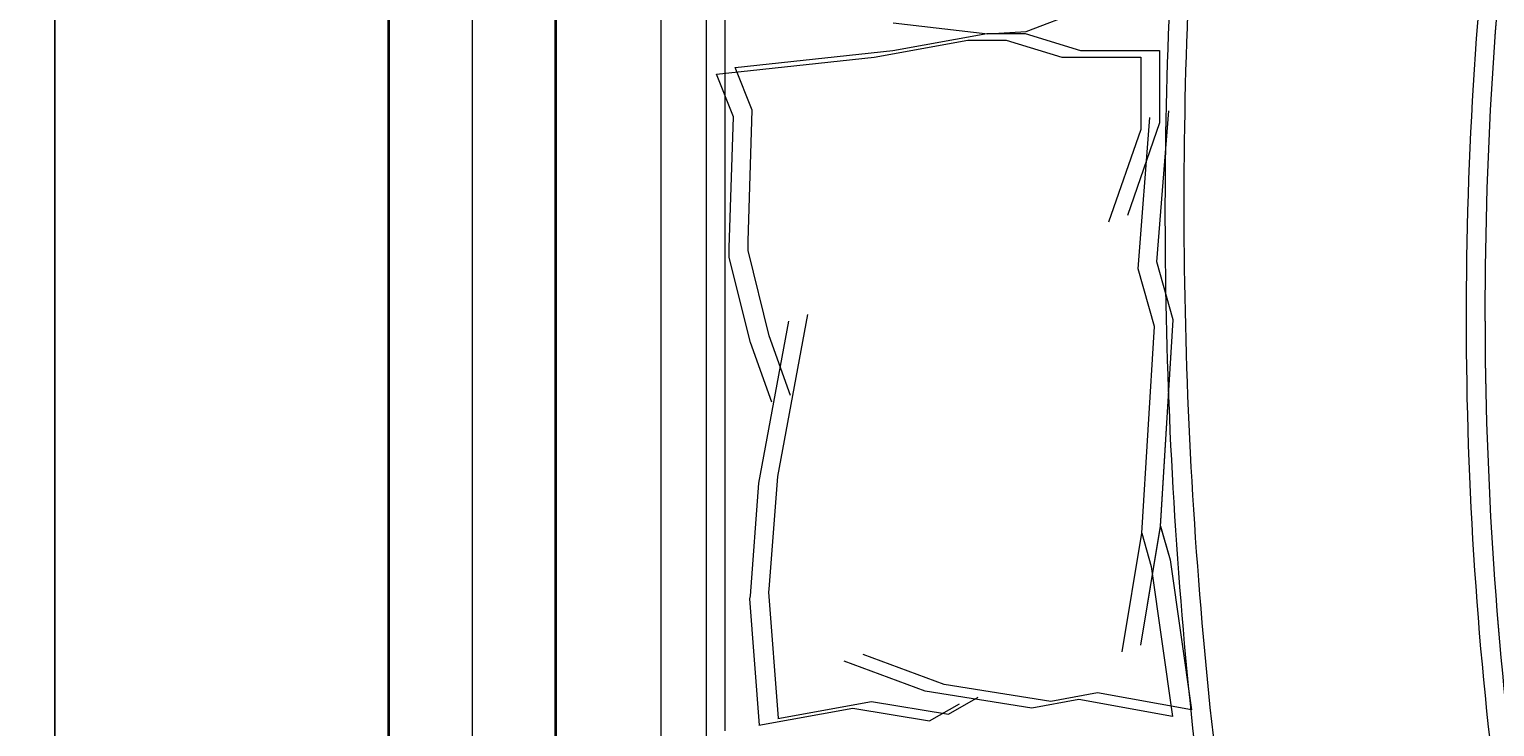
# Model space of a CAD drawing. Units: inches. Extents: x 1962 to 2771, y 1245 to 2660.
# Tile 25 of 114: x 2077 to 2116, y 1852 to 1871. Entities that reach past the tile are written whole.
import ezdxf

# ---------------------------------------------------------------- set-up
doc = ezdxf.new("R2010")
doc.units = ezdxf.units.IN
for name, color, linetype, lineweight in [('A-ANNO-DIMS', 2, 'Continuous', 18), ('A-FURN', 8, 'Continuous', 13), ('A-GLAZ', 4, 'Continuous', 18), ('A-WALL', 7, 'Continuous', 35)]:
    doc.layers.add(name, color=color, linetype=linetype, lineweight=lineweight)
doc.styles.get("Standard").update_dxf_attribs({"font": 'arial.ttf'})
doc.dimstyles.get("Standard").update_dxf_attribs({"dimtxt": 0.18, "dimasz": 0.18, "dimexe": 0.18, "dimexo": 0.0625, "dimgap": 0.09, "dimtad": 0, "dimtih": 1, "dimtoh": 1, "dimdec": 4, "dimzin": 0, "dimdsep": 46, "dimtxsty": 'Standard', "dimcen": 0.09, "dimadec": 0, "dimazin": 0, "dimtfac": 1, "dimtdec": 4, "dimtofl": 0, "dimtmove": 0, "dimatfit": 3, "dimfxl": 1, "dimtolj": 1, "dimtzin": 0, "dimarcsym": 0})

# ---------------------------------------------------------------- blocks, each defined once
blk = doc.blocks.new('BED-PLAN')
for p, q in [((0, 2.764), (0, 40.751)), ((1.219, 2.764), (1.219, 40.752)), ((1.219, 2.763), (1.219, 40.751)), ((1.727, 2.945), (1.727, 40.933)), ((1.727, 2.945), (1.727, 40.933)), ((9.838, 21.81), (11.301, 22.362)), ((9.838, 21.81), (11.301, 22.362)), ((6.247, 21.296), (8.776, 21.755)), ((6.247, 21.296), (8.776, 21.755)), ((6.254, 22.046), (8.806, 21.745)), ((6.254, 22.046), (8.806, 21.745)), ((8.776, 21.755), (9.81, 21.755)), ((8.776, 21.755), (9.81, 21.755)), ((8.806, 21.745), (9.838, 21.81)), ((8.806, 21.745), (9.838, 21.81)), ((9.81, 21.755), (11.304, 21.296)), ((9.81, 21.755), (11.304, 21.296)), ((5.739, 21.114), (8.268, 21.574)), ((5.739, 21.114), (8.268, 21.574)), ((8.268, 21.574), (9.302, 21.574)), ((8.268, 21.574), (9.302, 21.574)), ((9.302, 21.574), (10.796, 21.114)), ((9.302, 21.574), (10.796, 21.114)), ((1.487, 20.655), (5.739, 21.114)), ((1.487, 20.654), (5.739, 21.114)), ((1.995, 20.836), (6.247, 21.296)), ((1.995, 20.836), (6.247, 21.296)), ((10.796, 21.114), (12.927, 21.114)), ((10.796, 21.114), (12.927, 21.114)), ((11.304, 21.296), (13.436, 21.296)), ((11.304, 21.296), (13.436, 21.296)), ((12.927, 21.114), (12.927, 19.161)), ((12.927, 21.114), (12.927, 19.161)), ((13.436, 21.296), (13.436, 19.342)), ((13.436, 21.296), (13.436, 19.342)), ((1.946, 19.506), (1.487, 20.655)), ((1.946, 19.505), (1.487, 20.654)), ((2.455, 19.687), (1.995, 20.836)), ((2.455, 19.687), (1.995, 20.836)), ((1.831, 15.972), (1.946, 19.506)), ((1.831, 15.972), (1.946, 19.505)), ((2.34, 16.153), (2.455, 19.687)), ((2.34, 16.153), (2.455, 19.687)), ((12.853, 15.409), (13.173, 19.489)), ((12.853, 15.409), (13.173, 19.488)), ((13.361, 15.591), (13.682, 19.67)), ((13.361, 15.591), (13.682, 19.67)), ((12.927, 19.161), (12.06, 16.661)), ((12.927, 19.161), (12.06, 16.661)), ((13.436, 19.342), (12.568, 16.843)), ((13.436, 19.342), (12.568, 16.843)), ((1.831, 15.716), (1.831, 15.972)), ((1.831, 15.716), (1.831, 15.972)), ((2.34, 15.898), (2.34, 16.153)), ((2.34, 15.897), (2.34, 16.153)), ((2.914, 13.6), (2.34, 15.898)), ((2.914, 13.599), (2.34, 15.897)), ((2.406, 13.418), (1.831, 15.716)), ((2.406, 13.418), (1.831, 15.716)), ((13.296, 13.851), (12.853, 15.409)), ((13.296, 13.851), (12.853, 15.409)), ((13.804, 14.033), (13.361, 15.591)), ((13.804, 14.032), (13.361, 15.591)), ((2.636, 9.626), (3.44, 13.993)), ((2.636, 9.626), (3.44, 13.992)), ((3.144, 9.808), (3.949, 14.174)), ((3.144, 9.807), (3.949, 14.174)), ((12.953, 8.279), (13.296, 13.851)), ((12.953, 8.279), (13.296, 13.851)), ((13.461, 8.461), (13.804, 14.033)), ((13.461, 8.46), (13.804, 14.032)), ((3.489, 11.991), (2.914, 13.6)), ((3.489, 11.991), (2.914, 13.599)), ((2.981, 11.809), (2.406, 13.418)), ((2.981, 11.809), (2.406, 13.418)), ((2.406, 6.587), (2.636, 9.626)), ((2.406, 6.587), (2.636, 9.626)), ((2.914, 6.768), (3.144, 9.808)), ((2.914, 6.768), (3.144, 9.807)), ((12.931, 5.256), (13.461, 8.461)), ((12.931, 5.255), (13.461, 8.46)), ((13.461, 8.461), (13.718, 7.56)), ((13.461, 8.46), (13.718, 7.56)), ((12.423, 5.074), (12.953, 8.279)), ((12.423, 5.074), (12.953, 8.279)), ((12.953, 8.279), (13.21, 7.378)), ((12.953, 8.279), (13.21, 7.378)), ((13.718, 7.56), (14.292, 3.509)), ((13.718, 7.56), (14.292, 3.508)), ((13.21, 7.378), (13.784, 3.327)), ((13.21, 7.378), (13.784, 3.327)), ((2.9, 6.685), (2.914, 6.768)), ((2.9, 6.684), (2.914, 6.768)), ((2.392, 6.503), (2.406, 6.587)), ((2.392, 6.503), (2.406, 6.587)), ((2.653, 3.1), (2.392, 6.503)), ((2.653, 3.1), (2.392, 6.503)), ((3.162, 3.282), (2.9, 6.685)), ((3.162, 3.282), (2.9, 6.684)), ((7.118, 4.016), (4.935, 4.821)), ((7.118, 4.016), (4.935, 4.821)), ((7.626, 4.198), (5.443, 5.002)), ((7.626, 4.198), (5.443, 5.002)), ((9.991, 3.557), (7.118, 4.016)), ((9.992, 3.557), (7.118, 4.016)), ((10.5, 3.738), (7.626, 4.198)), ((10.5, 3.738), (7.626, 4.198)), ((11.764, 3.968), (10.5, 3.738)), ((11.764, 3.968), (10.5, 3.738)), ((14.292, 3.509), (11.764, 3.968)), ((14.292, 3.508), (11.764, 3.968)), ((2.636, 3.097), (5.164, 3.557)), ((2.636, 3.097), (5.164, 3.557)), ((3.144, 3.279), (5.673, 3.738)), ((3.144, 3.279), (5.673, 3.738)), ((5.164, 3.557), (7.233, 3.212)), ((5.164, 3.557), (7.233, 3.212)), ((5.673, 3.738), (7.741, 3.394)), ((5.673, 3.738), (7.741, 3.393)), ((7.233, 3.212), (8.038, 3.672)), ((7.233, 3.212), (8.038, 3.672)), ((7.741, 3.394), (8.546, 3.853)), ((7.741, 3.393), (8.546, 3.853)), ((11.256, 3.787), (9.991, 3.557)), ((11.256, 3.786), (9.992, 3.557)), ((13.784, 3.327), (11.256, 3.787)), ((13.784, 3.327), (11.256, 3.786))]:
    blk.add_line(p, q)
for centre, radius, start, end in [((124.762, 14.297), 102.556, 171.78449, 186.90062), ((124.762, 14.296), 102.556, 171.78449, 186.90062), ((124.254, 14.115), 102.556, 171.78449, 186.90062), ((124.254, 14.115), 102.556, 171.78449, 186.90062), ((145.219, 17.161), 131.131, 176.08655, 186.78213), ((145.219, 17.161), 131.131, 176.08655, 186.78213), ((144.711, 16.979), 131.131, 176.08655, 186.78213), ((144.711, 16.979), 131.131, 176.08655, 186.78213)]:
    blk.add_arc(centre, radius, start, end)
blk = doc.blocks.new('WIN-60IN-A')
blk.add_line((2.25, 60), (2.25, 0))
blk = doc.blocks.new('*D22')
at = {"layer": 'A-ANNO-DIMS', "color": 0, "lineweight": -2, "transparency": 16777216}
for p, q in [((2086.245, 1906.501), (2077.127, 1906.501)), ((2077.307, 1906.321), (2077.307, 1876.683)), ((2077.307, 1846.681), (2077.307, 1876.319)), ((2086.245, 1846.501), (2077.127, 1846.501))]:
    blk.add_line(p, q, dxfattribs=at)
at = {"layer": 'A-ANNO-DIMS', "color": 0, "transparency": 16777216}
for points in [[(2077.277, 1906.321), (2077.337, 1906.321), (2077.307, 1906.501)], [(2077.277, 1846.681), (2077.337, 1846.681), (2077.307, 1846.501)]]:
    blk.add_solid(points, dxfattribs=at)
at = {"layer": 'Defpoints', "color": 0, "transparency": 16777216}
for p in [(2077.307, 1906.501), (2086.307, 1906.501), (2086.307, 1846.501)]:
    blk.add_point(p, dxfattribs=at)
at = {"layer": 'A-ANNO-DIMS', "color": 0, "transparency": 16777216, "insert": (2077.307, 1876.501), "char_height": 0.18, "attachment_point": 5}
blk.add_mtext('\\A1;W3A 60 TYP.', dxfattribs=at)

msp = doc.modelspace()

# ---------------------------------------------------------------- linework, layer by layer
at = {"layer": 'A-WALL'}
for p, q in [((2086.3074, 1928.8437), (2086.3074, 1486.3437)), ((2090.8074, 1928.8437), (2090.8074, 1784.8437))]:
    msp.add_line(p, q, dxfattribs=at)

# ---------------------------------------------------------------- block references
at = {"layer": 'A-FURN'}
msp.add_blockref('BED-PLAN', (2093.6551, 1848.7344), dxfattribs=at)
at = {"layer": 'A-GLAZ'}
msp.add_blockref('WIN-60IN-A', (2086.3074, 1846.5013), dxfattribs=at)

# ---------------------------------------------------------------- dimensions: what is measured, and where the dimension line sits
at = {"layer": 'A-ANNO-DIMS'}
dim = msp.add_linear_dim(base=(2077.3074, 1906.5013), p1=(2086.3074, 1846.5013), p2=(2086.3074, 1906.5013), angle=90, text='W3A <> TYP.', dimstyle='Standard', override={"dimdec": 0, "dimlfac": 1, "dimrnd": 0, "dimzin": 0, "dimdsep": 46, "dimlunit": 2}, dxfattribs=at)
dim.commit()
dim.dimension.update_dxf_attribs({"geometry": '*D22', "text_midpoint": (2077.3074, 1876.5013)})

doc.saveas('drawing.dxf')
